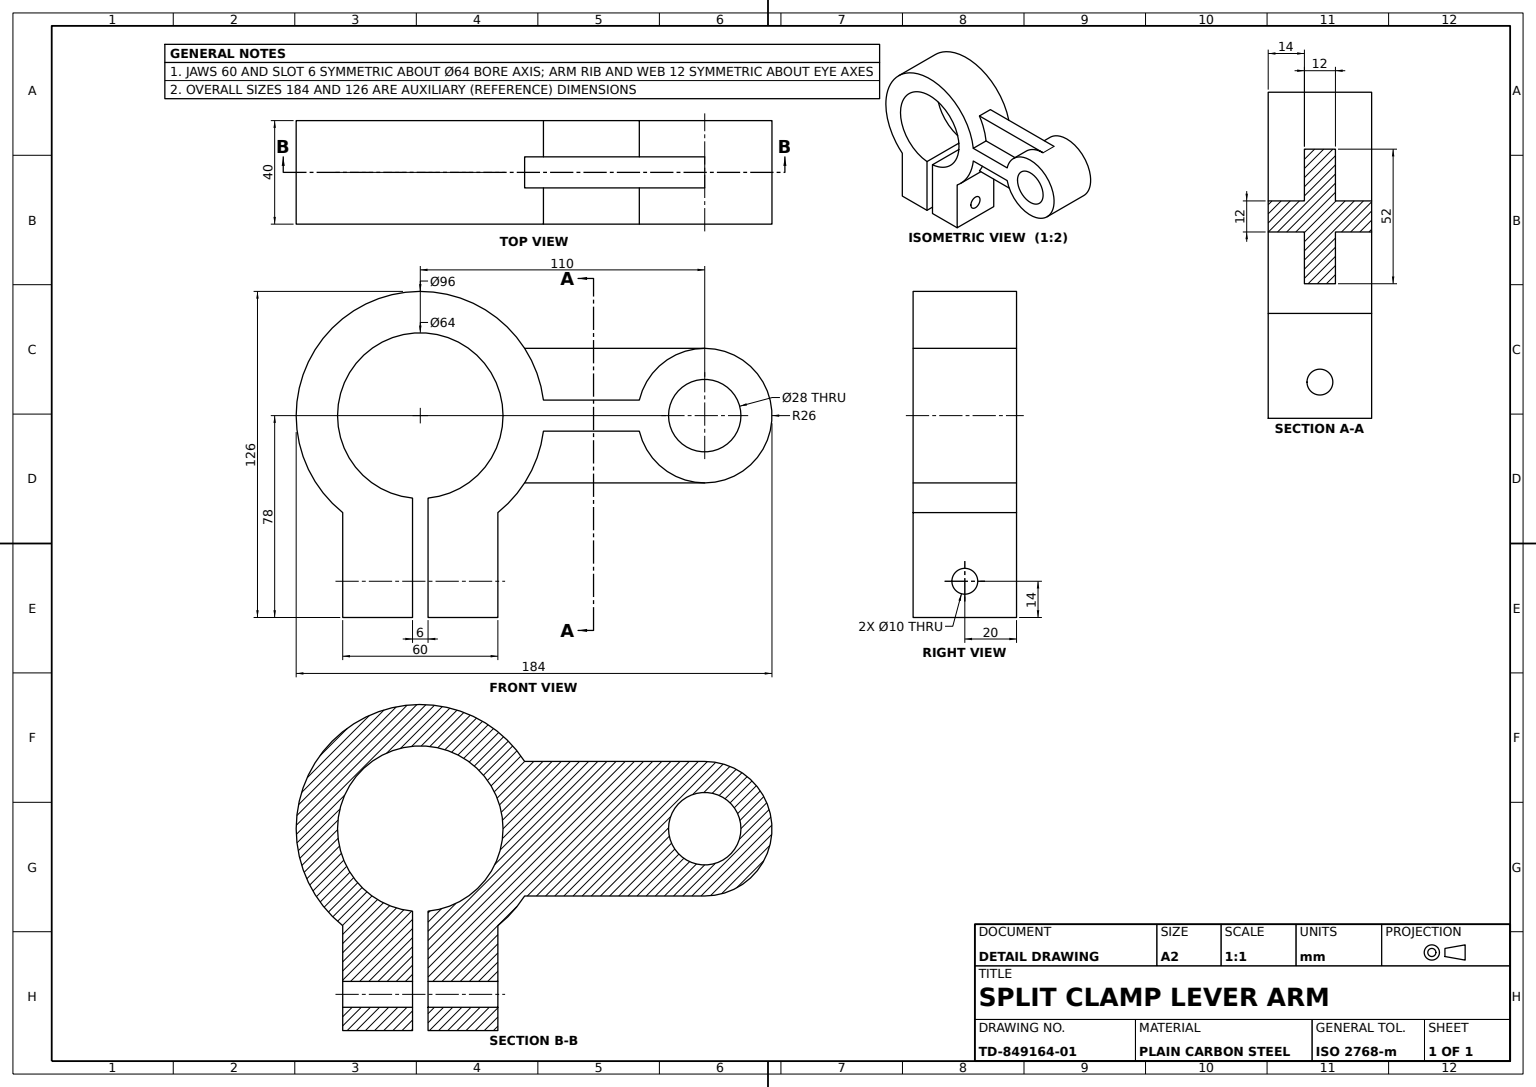
from build123d import *

# Parameters (mm, degrees)
CLAMP_EYE_96X40_DEPTH       = 20
ARM_AND_SMALL_EYE_PROFILE_R = 14
ARM_AND_SMALL_EYE_DEPTH     = 20
CLAMP_SCREW_HOLE_SKETCH_R   = 5
CLAMP_SCREW_HOLE_DEPTH      = 60
ARM_RIB_1_REACH             = 188.473
ARM_RIB_1_SKETCH_WALL_W     = 444.596554162
ARM_RIB_1_SKETCH_WALL_H     = 12
ARM_RIB_2_REACH             = 188.473
ARM_RIB_2_SKETCH_WALL_W     = 444.596554162
ARM_RIB_2_SKETCH_WALL_H     = 12


with BuildPart() as part:
    # Clamp Eye Profile → Clamp Eye Ø96x40 (new, symmetric)
    with BuildSketch(Plane.XY):
        with BuildLine():
            Line((-30, 40.53001201), (-30, 0))
            Line((-30, 0), (-3, 0))
            Line((-3, 0), (-3, 46.140935356))
            ThreePointArc((-3, 46.140935356), (0, 110), (3, 46.140935356))
            Line((3, 46.140935356), (3, 0))
            Line((3, 0), (30, 0))
            Line((30, 0), (30, 40.53001201))
            ThreePointArc((30, 40.53001201), (0, 126), (-30, 40.53001201))
        make_face()
    extrude(amount=CLAMP_EYE_96X40_DEPTH, both=True)

    # Arm and Small Eye Profile → Arm and Small Eye (add, symmetric)
    with BuildSketch(Plane.XY):
        with BuildLine():
            Line((47.623523599, 72), (84.701778719, 72))
            ThreePointArc((84.701778719, 72), (136, 78), (84.701778719, 84))
            Line((84.701778719, 84), (47.623523599, 84))
            ThreePointArc((47.623523599, 84), (48, 78), (47.623523599, 72))
        make_face()
        with Locations((110, 78)):
            Circle(ARM_AND_SMALL_EYE_PROFILE_R, mode=Mode.SUBTRACT)
    extrude(amount=ARM_AND_SMALL_EYE_DEPTH, both=True)

    # Clamp Screw Hole Sketch → Clamp Screw Hole (cut)
    with BuildSketch(Plane(origin=(30, 0, 0), x_dir=(0, 0, -1), z_dir=(1, 0, 0))):
        with Locations((0, 14)):
            Circle(CLAMP_SCREW_HOLE_SKETCH_R)
    extrude(amount=-CLAMP_SCREW_HOLE_DEPTH, mode=Mode.SUBTRACT)

    # Arm Rib 1 Sketch wall → Arm Rib 1 (add, up to next)
    with BuildSketch(Plane(origin=(75.174241002, 104, 0), x_dir=(-1, 0, 0), z_dir=(0, -1, 0)), mode=Mode.PRIVATE) as arm_rib_1_sk1:
        Rectangle(ARM_RIB_1_SKETCH_WALL_W, ARM_RIB_1_SKETCH_WALL_H)
    arm_rib_1_tool1 = extrude(arm_rib_1_sk1.sketch, amount=ARM_RIB_1_REACH, mode=Mode.PRIVATE) - part.part
    add(arm_rib_1_tool1.solids().sort_by_distance((75.174241002, 104, 0))[0])

    # Arm Rib 2 Sketch wall → Arm Rib 2 (add, up to next)
    with BuildSketch(Plane(origin=(75.174241002, 52, 0), x_dir=(-1, 0, 0), z_dir=(0, -1, 0)), mode=Mode.PRIVATE) as arm_rib_2_sk1:
        Rectangle(ARM_RIB_2_SKETCH_WALL_W, ARM_RIB_2_SKETCH_WALL_H)
    arm_rib_2_tool1 = extrude(arm_rib_2_sk1.sketch, amount=-ARM_RIB_2_REACH, mode=Mode.PRIVATE) - part.part
    add(arm_rib_2_tool1.solids().sort_by_distance((75.174241002, 52, 0))[0])


solid = part.part
